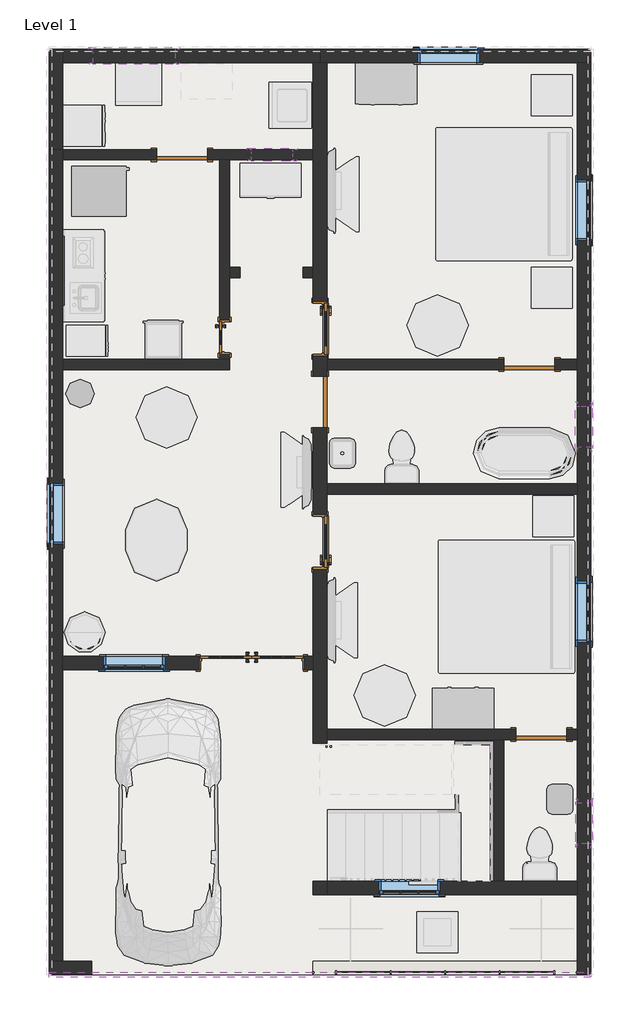
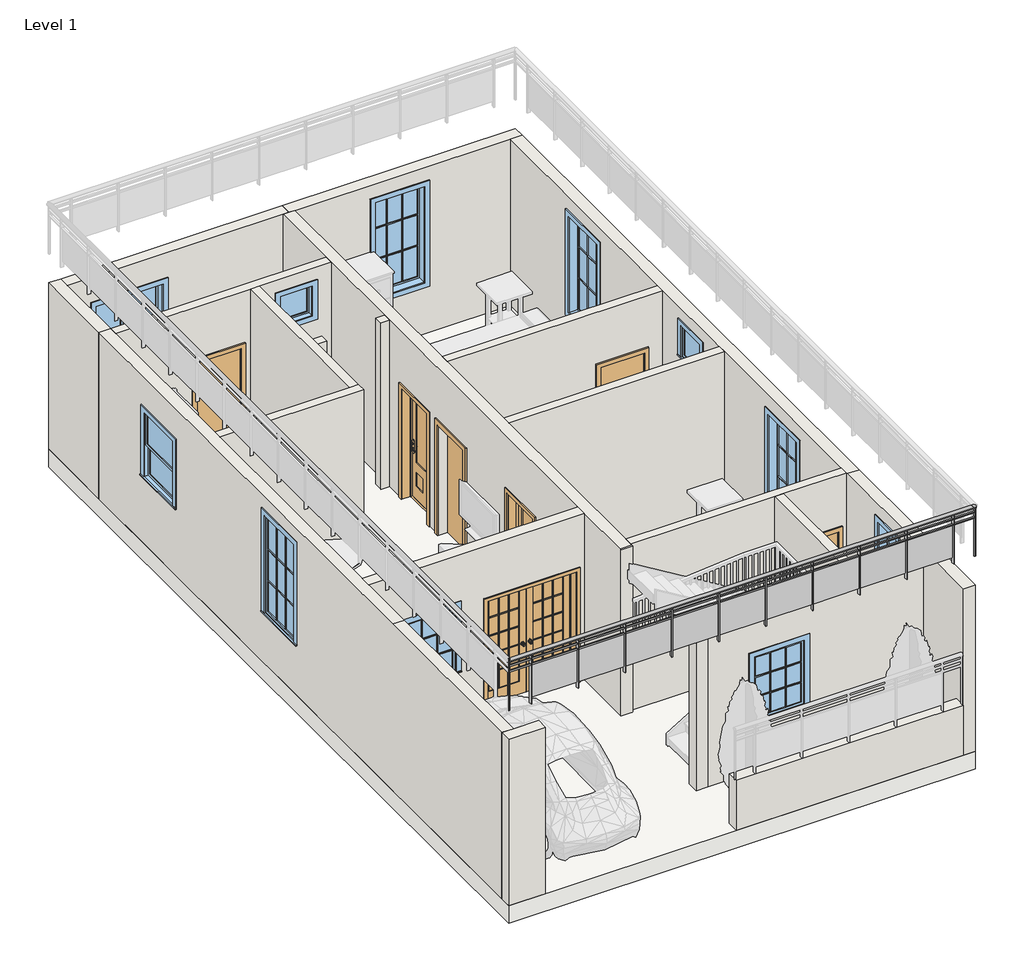
# One storey, part 1 of 3: 20 walls, 11 windows, 8 doors, 1 railing, 1 slab.
"""IFC4 building model written with IfcOpenShell, lengths in millimetres."""

from ifc_helpers import new_model, si_unit, point, frame, origin, origin_with_axes, place, context, project, spatial, polyline, ellipse_curve, trimmed, outline, extrude, faceted_brep, transform, mapped, element, save
from ifc_brep_helpers import plane_surface, extruded_surface, advanced_brep
from components import door_41326d50, door_ad59dcae, door_9d00318c, door_059bf842, door_059fdd7e, door_255cab33, door_53b1b562, window_29c06734, window_8b323df3, window_0862ab64, window_31198920, window_e41d21a6, window_3d781103

model = new_model("IFC4")

# Units and contexts
model_context = context("Model", 3, world=origin())
ifc_project = project(units=[si_unit("LENGTHUNIT", "METRE", prefix="MILLI")], contexts=[model_context])

# Site, building, storey
site = spatial("IfcSite", under=ifc_project)
building = spatial("IfcBuilding", under=site)
storey = spatial("IfcBuildingStorey", under=building, Name="Level 1", Elevation=0.0)

# Doors
placement = place(None, origin())
door_shape = door_41326d50(model_context)
element("IfcDoor", 1, ObjectType="30\" x 80\"", at=placement, inside=storey, context=model_context, shape_type="MappedRepresentation", body=[
    mapped(door_shape, transform((-8535.4123398, 7546.9033005, 0.0), x_axis=(0.0, 1.0, 0.0), y_axis=(-1.0, 0.0, 0.0), z_axis=(0.0, 0.0, 1.0))),
])
door_2_shape = door_ad59dcae(model_context)
element("IfcDoor", 2, ObjectType="30\" x 80\"", at=placement, inside=storey, context=model_context, shape_type="MappedRepresentation", body=[
    mapped(door_2_shape, transform((-8535.4123398, 4371.9033005, 0.0), x_axis=(0.0, -1.0, 0.0), y_axis=(1.0, 0.0, 0.0), z_axis=(0.0, 0.0, 1.0))),
])
door_3_shape = door_9d00318c(model_context)
element("IfcDoor", 3, ObjectType="Door-Interior-Double-Full Glass-Wood : 60\" x 80\"", at=placement, inside=storey, context=model_context, shape_type="MappedRepresentation", body=[
    mapped(door_3_shape, transform((-9554.5873398, 2571.6783005, 0.0), x_axis=(1.0, 0.0, 0.0), y_axis=(0.0, 1.0, 0.0), z_axis=(0.0, 0.0, 1.0))),
])
door_4_shape = door_059bf842(model_context)
element("IfcDoor", 4, ObjectType="Door-Interior-Single-Full Glass-Wood : 18\" x 80\"", at=placement, inside=storey, context=model_context, shape_type="MappedRepresentation", body=[
    mapped(door_4_shape, transform((-9964.1623398, 7419.9033005, 0.0), x_axis=(0.0, -1.0, 0.0), y_axis=(1.0, 0.0, 0.0), z_axis=(0.0, 0.0, 1.0))),
])
door_5_shape = door_059fdd7e(model_context)
element("IfcDoor", 5, ObjectType="Single-Flush : 30\" x 80\"", at=placement, inside=storey, context=model_context, shape_type="MappedRepresentation", body=[
    mapped(door_5_shape, transform((-5236.5873398, 1501.7033005, 0.0), x_axis=(-1.0, 0.0, 0.0), y_axis=(0.0, -1.0, 0.0), z_axis=(0.0, 0.0, 1.0))),
])
door_6_shape = door_255cab33(model_context)
element("IfcDoor", 6, ObjectType="Single-Flush : 30\" x 80\"", at=placement, inside=storey, context=model_context, shape_type="MappedRepresentation", body=[
    mapped(door_6_shape, transform((-5414.3873398, 7013.5033005, 0.0), x_axis=(1.0, 0.0, 0.0), y_axis=(0.0, 1.0, 0.0), z_axis=(0.0, 0.0, 1.0))),
])
element("IfcDoor", 7, ObjectType="Single-Flush : 30\" x 80\"", at=placement, inside=storey, context=model_context, shape_type="MappedRepresentation", body=[
    mapped(door_6_shape, transform((-10595.9873398, 10137.7033005, 0.0), x_axis=(1.0, 0.0, 0.0), y_axis=(0.0, 1.0, 0.0), z_axis=(0.0, 0.0, 1.0))),
])
door_7_shape = door_53b1b562(model_context)
element("IfcDoor", 8, ObjectType="Single-Flush : 30\" x 80\"", at=placement, inside=storey, context=model_context, shape_type="MappedRepresentation", body=[
    mapped(door_7_shape, transform((-8538.5873398, 6454.7033005, 0.0), x_axis=(0.0, 1.0, 0.0), y_axis=(-1.0, 0.0, 0.0), z_axis=(0.0, 0.0, 1.0))),
])

# Railing
element("IfcRailing", 9, ObjectType="Glass Panel - Bottom Fill", at=placement, inside=storey, context=model_context, shape_type="SolidModel", body=[
    advanced_brep(
    [(-12577.1873398, -2041.5966995, 4495.8), (-12577.1873398, -2117.7966995, 4495.8), (-4499.9873398, -2041.5966995, 4495.8), (-4499.9873398, -2117.7966995, 4495.8)],
    [
        (0, 1, ellipse_curve(frame((-12577.1873398, -2079.6966995, 4495.8), z_axis=(-1.0, 0.0, 0.0), x_axis=(0.0, -1.0, 0.0)), 38.1, 28.575)),
        (1, 0, ellipse_curve(frame((-12577.1873398, -2079.6966995, 4495.8), z_axis=(-1.0, 0.0, 0.0), x_axis=(0.0, -1.0, 0.0)), 38.1, 28.575)),
        (2, 3, ellipse_curve(frame((-4499.9873398, -2079.6966995, 4495.8), z_axis=(1.0, 0.0, 0.0), x_axis=(0.0, -1.0, 0.0)), 38.1, 28.575)),
        (3, 2, ellipse_curve(frame((-4499.9873398, -2079.6966995, 4495.8), z_axis=(1.0, 0.0, 0.0), x_axis=(0.0, -1.0, 0.0)), 38.1, 28.575)),
        (0, 2),
        (3, 1),
    ],
    [
        plane_surface(frame((-12577.1873398, -2079.6966995, 4495.8), z_axis=(-1.0, 0.0, 0.0), x_axis=(0.0, 1.0, 0.0))),
        plane_surface(frame((-4499.9873398, -2079.6966995, 4495.8), z_axis=(1.0, 0.0, 0.0), x_axis=(0.0, 1.0, 0.0))),
        extruded_surface(trimmed(ellipse_curve(frame((-4499.9873398, -2079.6966995, 4495.8), z_axis=(-1.0, 0.0, 0.0), x_axis=(0.0, -1.0, 0.0)), 38.1, 28.575), [point((-4499.9873398, -2041.5966995, 4495.8))], [point((-4499.9873398, -2117.7966995, 4495.8))], True, "CARTESIAN"), (-8077.200000000001, 0.0, 0.0), 8077.200000000001),
        extruded_surface(trimmed(ellipse_curve(frame((-4499.9873398, -2079.6966995, 4495.8), z_axis=(-1.0, 0.0, 0.0), x_axis=(0.0, -1.0, 0.0)), 38.1, 28.575), [point((-4499.9873398, -2117.7966995, 4495.8))], [point((-4499.9873398, -2041.5966995, 4495.8))], True, "CARTESIAN"), (-8077.200000000001, 0.0, 0.0), 8077.200000000001),
    ],
    [
        (0, [[1, 2]]),
        (1, [[3, 4]]),
        (2, [[-1, 5, -4, 6]]),
        (3, [[-2, -6, -3, -5]]),
    ],
),
    extrude(outline(polyline([(-12577.1873398, -2092.3966995), (-12577.1873398, -2066.9966995), (-4499.9873398, -2066.9966995), (-4499.9873398, -2092.3966995), (-12577.1873398, -2092.3966995)])), frame((0.0, 0.0, 4381.5), z_axis=(0.0, 0.0, 1.0), x_axis=(1.0, 0.0, 0.0)), (0.0, 0.0, 1.0), 25.4),
    extrude(outline(polyline([(-12577.1873398, -2092.3966995), (-12577.1873398, -2066.9966995), (-4499.9873398, -2066.9966995), (-4499.9873398, -2092.3966995), (-12577.1873398, -2092.3966995)])), frame((0.0, 0.0, 4279.9), z_axis=(0.0, 0.0, 1.0), x_axis=(1.0, 0.0, 0.0)), (0.0, 0.0, 1.0), 25.4),
    extrude(outline(polyline([(-4887.3373398, -2105.0966995), (-4887.3373398, -2054.2966995), (-4874.6373398, -2054.2966995), (-4874.6373398, -2105.0966995), (-4887.3373398, -2105.0966995)])), frame((0.0, 0.0, 3581.4), z_axis=(0.0, 0.0, 1.0), x_axis=(1.0, 0.0, 0.0)), (0.0, 0.0, 1.0), 885.6788223),
    extrude(outline(polyline([(-5693.7873398, -2073.1615425), (-4880.9873398, -2073.1615425), (-4880.9873398, -2079.5115425), (-5693.7873398, -2079.5115425), (-5693.7873398, -2073.1615425)])), frame((0.0, 0.0, 3683.0), z_axis=(0.0, 0.0, 1.0), x_axis=(1.0, 0.0, 0.0)), (0.0, 0.0, 1.0), 596.9),
    extrude(outline(polyline([(-5700.1373398, -2105.0966995), (-5700.1373398, -2054.2966995), (-5687.4373398, -2054.2966995), (-5687.4373398, -2105.0966995), (-5700.1373398, -2105.0966995)])), frame((0.0, 0.0, 3581.4), z_axis=(0.0, 0.0, 1.0), x_axis=(1.0, 0.0, 0.0)), (0.0, 0.0, 1.0), 885.6788223),
    extrude(outline(polyline([(-6506.5873398, -2073.1615425), (-5693.7873398, -2073.1615425), (-5693.7873398, -2079.5115425), (-6506.5873398, -2079.5115425), (-6506.5873398, -2073.1615425)])), frame((0.0, 0.0, 3683.0), z_axis=(0.0, 0.0, 1.0), x_axis=(1.0, 0.0, 0.0)), (0.0, 0.0, 1.0), 596.9),
    extrude(outline(polyline([(-6512.9373398, -2105.0966995), (-6512.9373398, -2054.2966995), (-6500.2373398, -2054.2966995), (-6500.2373398, -2105.0966995), (-6512.9373398, -2105.0966995)])), frame((0.0, 0.0, 3581.4), z_axis=(0.0, 0.0, 1.0), x_axis=(1.0, 0.0, 0.0)), (0.0, 0.0, 1.0), 885.6788223),
    extrude(outline(polyline([(-7319.3873398, -2073.1615425), (-6506.5873398, -2073.1615425), (-6506.5873398, -2079.5115425), (-7319.3873398, -2079.5115425), (-7319.3873398, -2073.1615425)])), frame((0.0, 0.0, 3683.0), z_axis=(0.0, 0.0, 1.0), x_axis=(1.0, 0.0, 0.0)), (0.0, 0.0, 1.0), 596.9),
    extrude(outline(polyline([(-7325.7373398, -2105.0966995), (-7325.7373398, -2054.2966995), (-7313.0373398, -2054.2966995), (-7313.0373398, -2105.0966995), (-7325.7373398, -2105.0966995)])), frame((0.0, 0.0, 3581.4), z_axis=(0.0, 0.0, 1.0), x_axis=(1.0, 0.0, 0.0)), (0.0, 0.0, 1.0), 885.6788223),
    extrude(outline(polyline([(-8132.1873398, -2073.1615425), (-7319.3873398, -2073.1615425), (-7319.3873398, -2079.5115425), (-8132.1873398, -2079.5115425), (-8132.1873398, -2073.1615425)])), frame((0.0, 0.0, 3683.0), z_axis=(0.0, 0.0, 1.0), x_axis=(1.0, 0.0, 0.0)), (0.0, 0.0, 1.0), 596.9),
    extrude(outline(polyline([(-8138.5373398, -2105.0966995), (-8138.5373398, -2054.2966995), (-8125.8373398, -2054.2966995), (-8125.8373398, -2105.0966995), (-8138.5373398, -2105.0966995)])), frame((0.0, 0.0, 3581.4), z_axis=(0.0, 0.0, 1.0), x_axis=(1.0, 0.0, 0.0)), (0.0, 0.0, 1.0), 885.6788223),
    extrude(outline(polyline([(-8944.9873398, -2073.1615425), (-8132.1873398, -2073.1615425), (-8132.1873398, -2079.5115425), (-8944.9873398, -2079.5115425), (-8944.9873398, -2073.1615425)])), frame((0.0, 0.0, 3683.0), z_axis=(0.0, 0.0, 1.0), x_axis=(1.0, 0.0, 0.0)), (0.0, 0.0, 1.0), 596.9),
    extrude(outline(polyline([(-8951.3373398, -2105.0966995), (-8951.3373398, -2054.2966995), (-8938.6373398, -2054.2966995), (-8938.6373398, -2105.0966995), (-8951.3373398, -2105.0966995)])), frame((0.0, 0.0, 3581.4), z_axis=(0.0, 0.0, 1.0), x_axis=(1.0, 0.0, 0.0)), (0.0, 0.0, 1.0), 885.6788223),
    extrude(outline(polyline([(-9757.7873398, -2073.1615425), (-8944.9873398, -2073.1615425), (-8944.9873398, -2079.5115425), (-9757.7873398, -2079.5115425), (-9757.7873398, -2073.1615425)])), frame((0.0, 0.0, 3683.0), z_axis=(0.0, 0.0, 1.0), x_axis=(1.0, 0.0, 0.0)), (0.0, 0.0, 1.0), 596.9),
    extrude(outline(polyline([(-9764.1373398, -2105.0966995), (-9764.1373398, -2054.2966995), (-9751.4373398, -2054.2966995), (-9751.4373398, -2105.0966995), (-9764.1373398, -2105.0966995)])), frame((0.0, 0.0, 3581.4), z_axis=(0.0, 0.0, 1.0), x_axis=(1.0, 0.0, 0.0)), (0.0, 0.0, 1.0), 885.6788223),
    extrude(outline(polyline([(-10570.5873398, -2073.1615425), (-9757.7873398, -2073.1615425), (-9757.7873398, -2079.5115425), (-10570.5873398, -2079.5115425), (-10570.5873398, -2073.1615425)])), frame((0.0, 0.0, 3683.0), z_axis=(0.0, 0.0, 1.0), x_axis=(1.0, 0.0, 0.0)), (0.0, 0.0, 1.0), 596.9),
    extrude(outline(polyline([(-10576.9373398, -2105.0966995), (-10576.9373398, -2054.2966995), (-10564.2373398, -2054.2966995), (-10564.2373398, -2105.0966995), (-10576.9373398, -2105.0966995)])), frame((0.0, 0.0, 3581.4), z_axis=(0.0, 0.0, 1.0), x_axis=(1.0, 0.0, 0.0)), (0.0, 0.0, 1.0), 885.6788223),
    extrude(outline(polyline([(-11383.3873398, -2073.1615425), (-10570.5873398, -2073.1615425), (-10570.5873398, -2079.5115425), (-11383.3873398, -2079.5115425), (-11383.3873398, -2073.1615425)])), frame((0.0, 0.0, 3683.0), z_axis=(0.0, 0.0, 1.0), x_axis=(1.0, 0.0, 0.0)), (0.0, 0.0, 1.0), 596.9),
    extrude(outline(polyline([(-11389.7373398, -2105.0966995), (-11389.7373398, -2054.2966995), (-11377.0373398, -2054.2966995), (-11377.0373398, -2105.0966995), (-11389.7373398, -2105.0966995)])), frame((0.0, 0.0, 3581.4), z_axis=(0.0, 0.0, 1.0), x_axis=(1.0, 0.0, 0.0)), (0.0, 0.0, 1.0), 885.6788223),
    extrude(outline(polyline([(-12196.1873398, -2073.1615425), (-11383.3873398, -2073.1615425), (-11383.3873398, -2079.5115425), (-12196.1873398, -2079.5115425), (-12196.1873398, -2073.1615425)])), frame((0.0, 0.0, 3683.0), z_axis=(0.0, 0.0, 1.0), x_axis=(1.0, 0.0, 0.0)), (0.0, 0.0, 1.0), 596.9),
    extrude(outline(polyline([(-12202.5373398, -2105.0966995), (-12202.5373398, -2054.2966995), (-12189.8373398, -2054.2966995), (-12189.8373398, -2105.0966995), (-12202.5373398, -2105.0966995)])), frame((0.0, 0.0, 3581.4), z_axis=(0.0, 0.0, 1.0), x_axis=(1.0, 0.0, 0.0)), (0.0, 0.0, 1.0), 885.6788223),
    extrude(outline(polyline([(-4512.6873398, -2089.2216995), (-4512.6873398, -2070.1716995), (-4493.6373398, -2070.1716995), (-4493.6373398, -2089.2216995), (-4512.6873398, -2089.2216995)])), frame((0.0, 0.0, 3581.4), z_axis=(0.0, 0.0, 1.0), x_axis=(1.0, 0.0, 0.0)), (0.0, 0.0, 1.0), 885.6788223),
    extrude(outline(polyline([(-12583.5373398, -2089.2216995), (-12583.5373398, -2070.1716995), (-12564.4873398, -2070.1716995), (-12564.4873398, -2089.2216995), (-12583.5373398, -2089.2216995)])), frame((0.0, 0.0, 3581.4), z_axis=(0.0, 0.0, 1.0), x_axis=(1.0, 0.0, 0.0)), (0.0, 0.0, 1.0), 885.6788223),
])

# Slab
element("IfcSlab", 10, at=placement, inside=storey, context=model_context, shape_type="SweptSolid", body=[
    extrude(outline(polyline([(-4499.9873398, 11712.5033005), (-4499.9873398, -2079.6966995), (-12577.1873398, -2079.6966995), (-12577.1873398, 11712.5033005), (-4499.9873398, 11712.5033005)])), frame((0.0, 0.0, -323.85), z_axis=(0.0, 0.0, 1.0), x_axis=(1.0, 0.0, 0.0)), (0.0, 0.0, 1.0), 323.85),
])

# Walls
element("IfcWall", 11, ObjectType="Generic - 8\"", at=placement, inside=storey, context=model_context, shape_type="Brep", body=[
    faceted_brep([(-4703.1873398, 11509.3033005, 0.0), (-4703.1873398, 7089.7033005, 0.0), (-4703.1873398, 6937.3033005, 0.0), (-4703.1873398, 5235.5033005, 0.0), (-4703.1873398, 5083.1033005, 0.0), (-4703.1873398, 1577.9033005, 0.0), (-4703.1873398, 1425.5033005, 0.0), (-4703.1873398, -682.6966995, 0.0), (-4703.1873398, -885.8966995, 0.0), (-4703.1873398, -1876.4966995, 0.0), (-4703.1873398, -2079.6966995, 0.0), (-4703.1873398, -2079.6966995, 914.4), (-4703.1873398, -2079.6966995, 3048.0), (-4703.1873398, -885.8966995, 3048.0), (-4703.1873398, -682.6966995, 3048.0), (-4703.1873398, 1400.1033005, 3048.0), (-4703.1873398, 1425.5033005, 3048.0), (-4703.1873398, 1577.9033005, 3048.0), (-4703.1873398, 5083.1033005, 3048.0), (-4703.1873398, 5235.5033005, 3048.0), (-4703.1873398, 6937.3033005, 3048.0), (-4703.1873398, 7089.7033005, 3048.0), (-4703.1873398, 11509.3033005, 3048.0), (-4703.1873398, 2873.3033005, 2743.2), (-4703.1873398, 2873.3033005, 914.4), (-4703.1873398, 3787.7033005, 914.4), (-4703.1873398, 3787.7033005, 2743.2), (-4703.1873398, 8855.0033005, 2743.2), (-4703.1873398, 8855.0033005, 914.4), (-4703.1873398, 9769.4033005, 914.4), (-4703.1873398, 9769.4033005, 2743.2), (-4703.1873398, -123.8966995, 2768.6), (-4703.1873398, -123.8966995, 2159.0), (-4703.1873398, 485.7033005, 2159.0), (-4703.1873398, 485.7033005, 2768.6), (-4703.1873398, 6391.2033005, 2768.6), (-4703.1873398, 5781.6033005, 2768.6), (-4703.1873398, 5781.6033005, 2159.0), (-4703.1873398, 6391.2033005, 2159.0), (-4499.9873398, 11509.3033005, 0.0), (-4499.9873398, 11509.3033005, 3048.0), (-4499.9873398, 1400.1033005, 3048.0), (-4499.9873398, -2079.6966995, 3048.0), (-4499.9873398, -2079.6966995, 0.0), (-4499.9873398, 2873.3033005, 2743.2), (-4499.9873398, 3787.7033005, 2743.2), (-4499.9873398, 3787.7033005, 914.4), (-4499.9873398, 2873.3033005, 914.4), (-4499.9873398, 8855.0033005, 2743.2), (-4499.9873398, 9769.4033005, 2743.2), (-4499.9873398, 9769.4033005, 914.4), (-4499.9873398, 8855.0033005, 914.4), (-4499.9873398, -123.8966995, 2768.6), (-4499.9873398, 485.7033005, 2768.6), (-4499.9873398, 485.7033005, 2159.0), (-4499.9873398, -123.8966995, 2159.0), (-4499.9873398, 6391.2033005, 2768.6), (-4499.9873398, 6391.2033005, 2159.0), (-4499.9873398, 5781.6033005, 2159.0), (-4499.9873398, 5781.6033005, 2768.6)], [[[0, 1, 2, 3, 4, 5, 6, 7, 8, 9, 10, 11, 12, 13, 14, 15, 16, 17, 18, 19, 20, 21, 22], [23, 24, 25, 26], [27, 28, 29, 30], [31, 32, 33, 34], [35, 36, 37, 38]], [[39, 40, 41, 42, 43], [44, 45, 46, 47], [48, 49, 50, 51], [52, 53, 54, 55], [56, 57, 58, 59]], [[10, 9, 8, 7, 6, 5, 4, 3, 2, 1, 0, 39, 43]], [[0, 22, 40, 39]], [[12, 11, 10, 43, 42]], [[15, 14, 13, 12, 42, 41]], [[22, 21, 20, 19, 18, 17, 16, 15, 41, 40]], [[24, 23, 44, 47]], [[25, 24, 47, 46]], [[26, 25, 46, 45]], [[23, 26, 45, 44]], [[28, 27, 48, 51]], [[29, 28, 51, 50]], [[30, 29, 50, 49]], [[27, 30, 49, 48]], [[32, 31, 52, 55]], [[33, 32, 55, 54]], [[34, 33, 54, 53]], [[31, 34, 53, 52]], [[57, 56, 35, 38]], [[58, 57, 38, 37]], [[59, 58, 37, 36]], [[56, 59, 36, 35]]]),
])
element("IfcWall", 12, ObjectType="Generic - 8\"", at=placement, inside=storey, context=model_context, shape_type="SweptSolid", body=[
    extrude(outline(polyline([(-8640.1873398, -1876.4966995), (-4703.1873398, -1876.4966995), (-4703.1873398, -2079.6966995), (-8640.1873398, -2079.6966995), (-8640.1873398, -1876.4966995)])), origin_with_axes(), (0.0, 0.0, 1.0), 914.4),
])
element("IfcWall", 13, ObjectType="Generic - 8\"", at=placement, inside=storey, context=model_context, shape_type="Brep", body=[
    faceted_brep([(-12373.9873398, -1876.4966995, 0.0), (-12373.9873398, 2466.9033005, 0.0), (-12373.9873398, 2670.1033005, 0.0), (-12373.9873398, 6937.3033005, 0.0), (-12373.9873398, 7089.7033005, 0.0), (-12373.9873398, 10061.5033005, 0.0), (-12373.9873398, 10213.9033005, 0.0), (-12373.9873398, 10213.9033005, 3048.0), (-12373.9873398, 10061.5033005, 3048.0), (-12373.9873398, 7089.7033005, 3048.0), (-12373.9873398, 6937.3033005, 3048.0), (-12373.9873398, 2670.1033005, 3048.0), (-12373.9873398, 2466.9033005, 3048.0), (-12373.9873398, 1400.1033005, 3048.0), (-12373.9873398, -1876.4966995, 3048.0), (-12373.9873398, 5248.2033005, 2743.2), (-12373.9873398, 5248.2033005, 914.4), (-12373.9873398, 4333.8033005, 914.4), (-12373.9873398, 4333.8033005, 2743.2), (-12373.9873398, 8867.7033005, 2438.4), (-12373.9873398, 8867.7033005, 1219.2), (-12373.9873398, 7953.3033005, 1219.2), (-12373.9873398, 7953.3033005, 2438.4), (-12577.1873398, -1876.4966995, 0.0), (-12577.1873398, -1876.4966995, 3048.0), (-12577.1873398, 1400.1033005, 3048.0), (-12577.1873398, 10213.9033005, 3048.0), (-12577.1873398, 10213.9033005, 0.0), (-12577.1873398, 5248.2033005, 2743.2), (-12577.1873398, 4333.8033005, 2743.2), (-12577.1873398, 4333.8033005, 914.4), (-12577.1873398, 5248.2033005, 914.4), (-12577.1873398, 8867.7033005, 2438.4), (-12577.1873398, 7953.3033005, 2438.4), (-12577.1873398, 7953.3033005, 1219.2), (-12577.1873398, 8867.7033005, 1219.2)], [[[0, 1, 2, 3, 4, 5, 6, 7, 8, 9, 10, 11, 12, 13, 14], [15, 16, 17, 18], [19, 20, 21, 22]], [[23, 24, 25, 26, 27], [28, 29, 30, 31], [32, 33, 34, 35]], [[6, 5, 4, 3, 2, 1, 0, 23, 27]], [[7, 6, 27, 26]], [[0, 14, 24, 23]], [[14, 13, 25, 24]], [[13, 12, 11, 10, 9, 8, 7, 26, 25]], [[16, 15, 28, 31]], [[17, 16, 31, 30]], [[18, 17, 30, 29]], [[15, 18, 29, 28]], [[20, 19, 32, 35]], [[21, 20, 35, 34]], [[22, 21, 34, 33]], [[19, 22, 33, 32]]]),
])
element("IfcWall", 14, ObjectType="Generic - 8\"", at=placement, inside=storey, context=model_context, shape_type="Brep", body=[
    faceted_brep([(-8640.1873398, 1374.7033005, 0.0), (-8640.1873398, 1374.7033005, 3048.0), (-8640.1873398, 1400.1033005, 3048.0), (-8640.1873398, 2466.9033005, 3048.0), (-8640.1873398, 2670.1033005, 3048.0), (-8640.1873398, 8308.9033005, 3048.0), (-8640.1873398, 8461.3033005, 3048.0), (-8640.1873398, 10061.5033005, 3048.0), (-8640.1873398, 10213.9033005, 3048.0), (-8640.1873398, 11509.3033005, 3048.0), (-8640.1873398, 11509.3033005, 0.0), (-8640.1873398, 10213.9033005, 0.0), (-8640.1873398, 10061.5033005, 0.0), (-8640.1873398, 8461.3033005, 0.0), (-8640.1873398, 8308.9033005, 0.0), (-8640.1873398, 7953.3033005, 0.0), (-8640.1873398, 7953.3033005, 2057.4), (-8640.1873398, 7140.5033005, 2057.4), (-8640.1873398, 7140.5033005, 0.0), (-8640.1873398, 6835.7033005, 0.0), (-8640.1873398, 6835.7033005, 2032.0), (-8640.1873398, 6073.7033005, 2032.0), (-8640.1873398, 6073.7033005, 0.0), (-8640.1873398, 4778.3033005, 0.0), (-8640.1873398, 4778.3033005, 2057.4), (-8640.1873398, 3965.5033005, 2057.4), (-8640.1873398, 3965.5033005, 0.0), (-8640.1873398, 2670.1033005, 0.0), (-8640.1873398, 2466.9033005, 0.0), (-8436.9873398, 1374.7033005, 3048.0), (-8436.9873398, 1374.7033005, 0.0), (-8436.9873398, 1425.5033005, 0.0), (-8436.9873398, 1577.9033005, 0.0), (-8436.9873398, 3965.5033005, 0.0), (-8436.9873398, 3965.5033005, 2057.4), (-8436.9873398, 4778.3033005, 2057.4), (-8436.9873398, 4778.3033005, 0.0), (-8436.9873398, 5083.1033005, 0.0), (-8436.9873398, 5235.5033005, 0.0), (-8436.9873398, 6073.7033005, 0.0), (-8436.9873398, 6073.7033005, 2032.0), (-8436.9873398, 6835.7033005, 2032.0), (-8436.9873398, 6835.7033005, 0.0), (-8436.9873398, 6937.3033005, 0.0), (-8436.9873398, 7089.7033005, 0.0), (-8436.9873398, 7140.5033005, 0.0), (-8436.9873398, 7140.5033005, 2057.4), (-8436.9873398, 7953.3033005, 2057.4), (-8436.9873398, 7953.3033005, 0.0), (-8436.9873398, 11509.3033005, 0.0), (-8436.9873398, 11509.3033005, 3048.0), (-8436.9873398, 7089.7033005, 3048.0), (-8436.9873398, 6937.3033005, 3048.0), (-8436.9873398, 5235.5033005, 3048.0), (-8436.9873398, 5083.1033005, 3048.0), (-8436.9873398, 1577.9033005, 3048.0), (-8436.9873398, 1425.5033005, 3048.0), (-8436.9873398, 1400.1033005, 3048.0), (-8538.5873398, 11509.3033005, 0.0), (-8538.5873398, 11509.3033005, 3048.0)], [[[0, 1, 2, 3, 4, 5, 6, 7, 8, 9, 10, 11, 12, 13, 14, 15, 16, 17, 18, 19, 20, 21, 22, 23, 24, 25, 26, 27, 28]], [[29, 30, 31, 32, 33, 34, 35, 36, 37, 38, 39, 40, 41, 42, 43, 44, 45, 46, 47, 48, 49, 50, 51, 52, 53, 54, 55, 56, 57]], [[30, 0, 28, 27, 26, 33, 32, 31]], [[48, 15, 14, 13, 12, 11, 10, 58, 49]], [[18, 45, 44, 43, 42, 19]], [[22, 39, 38, 37, 36, 23]], [[1, 0, 30, 29]], [[1, 29, 57, 2]], [[9, 8, 7, 6, 5, 4, 3, 2, 57, 56, 55, 54, 53, 52, 51, 50, 59]], [[47, 16, 15, 48]], [[16, 47, 46, 17]], [[17, 46, 45, 18]], [[20, 19, 42, 41]], [[21, 20, 41, 40]], [[22, 21, 40, 39]], [[10, 9, 59, 50, 49, 58]], [[25, 34, 33, 26]], [[34, 25, 24, 35]], [[35, 24, 23, 36]]]),
])
element("IfcWall", 15, ObjectType="Generic - 8\"", at=placement, inside=storey, context=model_context, shape_type="Brep", body=[
    faceted_brep([(-4703.1873398, -682.6966995, 0.0), (-5795.3873398, -682.6966995, 0.0), (-5947.7873398, -682.6966995, 0.0), (-8436.9873398, -682.6966995, 0.0), (-8436.9873398, -682.6966995, 3048.0), (-5947.7873398, -682.6966995, 3048.0), (-5795.3873398, -682.6966995, 3048.0), (-4703.1873398, -682.6966995, 3048.0), (-7662.2873398, -682.6966995, 2133.6), (-7662.2873398, -682.6966995, 914.4), (-6747.8873398, -682.6966995, 914.4), (-6747.8873398, -682.6966995, 2133.6), (-4703.1873398, -885.8966995, 0.0), (-4703.1873398, -885.8966995, 3048.0), (-8436.9873398, -885.8966995, 3048.0), (-8436.9873398, -885.8966995, 0.0), (-7662.2873398, -885.8966995, 2133.6), (-6747.8873398, -885.8966995, 2133.6), (-6747.8873398, -885.8966995, 914.4), (-7662.2873398, -885.8966995, 914.4)], [[[0, 1, 2, 3, 4, 5, 6, 7], [8, 9, 10, 11]], [[12, 13, 14, 15], [16, 17, 18, 19]], [[3, 2, 1, 0, 12, 15]], [[0, 7, 13, 12]], [[4, 3, 15, 14]], [[7, 6, 5, 4, 14, 13]], [[9, 8, 16, 19]], [[10, 9, 19, 18]], [[11, 10, 18, 17]], [[8, 11, 17, 16]]]),
])
element("IfcWall", 16, ObjectType="Generic - 8\"", at=placement, inside=storey, context=model_context, shape_type="SweptSolid", body=[
    extrude(outline(polyline([(3048.0, -12373.9873398), (0.0, -12373.9873398), (0.0, -10341.9873398), (2057.4, -10341.9873398), (2057.4, -8767.1873398), (0.0, -8767.1873398), (0.0, -8640.1873398), (3048.0, -8640.1873398), (3048.0, -12373.9873398)]), holes=[polyline([(2133.6, -11764.3873398), (2133.6, -10849.9873398), (914.4, -10849.9873398), (914.4, -11764.3873398), (2133.6, -11764.3873398)])]), frame((0.0, 2466.9033005, 0.0), z_axis=(0.0, 1.0, 0.0), x_axis=(0.0, 0.0, 1.0)), (0.0, 0.0, 1.0), 203.2),
])
element("IfcWall", 17, ObjectType="Generic - 8\"", at=placement, inside=storey, context=model_context, shape_type="SweptSolid", body=[
    extrude(outline(polyline([(-8640.1873398, -885.8966995), (-8640.1873398, -682.6966995), (-8436.9873398, -682.6966995), (-8436.9873398, -885.8966995), (-8640.1873398, -885.8966995)])), origin_with_axes(), (0.0, 0.0, 1.0), 3048.0),
])
element("IfcWall", 18, ObjectType="Generic - 8\"", at=placement, inside=storey, context=model_context, shape_type="Brep", body=[
    faceted_brep([(-12373.9873398, 11509.3033005, 0.0), (-8640.1873398, 11509.3033005, 0.0), (-8538.5873398, 11509.3033005, 0.0), (-8538.5873398, 11509.3033005, 3048.0), (-8640.1873398, 11509.3033005, 3048.0), (-12373.9873398, 11509.3033005, 3048.0), (-10697.5873398, 11509.3033005, 2540.0), (-10697.5873398, 11509.3033005, 1320.8), (-11916.7873398, 11509.3033005, 1320.8), (-11916.7873398, 11509.3033005, 2540.0), (-12373.9873398, 11712.5033005, 0.0), (-12373.9873398, 11712.5033005, 3048.0), (-8538.5873398, 11712.5033005, 3048.0), (-8538.5873398, 11712.5033005, 0.0), (-10697.5873398, 11712.5033005, 2540.0), (-11916.7873398, 11712.5033005, 2540.0), (-11916.7873398, 11712.5033005, 1320.8), (-10697.5873398, 11712.5033005, 1320.8)], [[[0, 1, 2, 3, 4, 5], [6, 7, 8, 9]], [[10, 11, 12, 13], [14, 15, 16, 17]], [[2, 1, 0, 10, 13]], [[3, 2, 13, 12]], [[5, 4, 3, 12, 11]], [[0, 5, 11, 10]], [[7, 6, 14, 17]], [[8, 7, 17, 16]], [[9, 8, 16, 15]], [[6, 9, 15, 14]]]),
])
element("IfcWall", 19, ObjectType="Generic - 8\"", at=placement, inside=storey, context=model_context, shape_type="Brep", body=[
    faceted_brep([(-8538.5873398, 11509.3033005, 0.0), (-8436.9873398, 11509.3033005, 0.0), (-4703.1873398, 11509.3033005, 0.0), (-4499.9873398, 11509.3033005, 0.0), (-4499.9873398, 11509.3033005, 3048.0), (-4703.1873398, 11509.3033005, 3048.0), (-8436.9873398, 11509.3033005, 3048.0), (-8538.5873398, 11509.3033005, 3048.0), (-6163.6873398, 11509.3033005, 2743.2), (-6163.6873398, 11509.3033005, 914.4), (-7078.0873398, 11509.3033005, 914.4), (-7078.0873398, 11509.3033005, 2743.2), (-8538.5873398, 11712.5033005, 0.0), (-8538.5873398, 11712.5033005, 3048.0), (-4499.9873398, 11712.5033005, 3048.0), (-4499.9873398, 11712.5033005, 0.0), (-6163.6873398, 11712.5033005, 2743.2), (-7078.0873398, 11712.5033005, 2743.2), (-7078.0873398, 11712.5033005, 914.4), (-6163.6873398, 11712.5033005, 914.4)], [[[0, 1, 2, 3, 4, 5, 6, 7], [8, 9, 10, 11]], [[12, 13, 14, 15], [16, 17, 18, 19]], [[3, 2, 1, 0, 12, 15]], [[0, 7, 13, 12]], [[4, 3, 15, 14]], [[7, 6, 5, 4, 14, 13]], [[8, 11, 17, 16]], [[11, 10, 18, 17]], [[10, 9, 19, 18]], [[9, 8, 16, 19]]]),
])
element("IfcWall", 20, ObjectType="Generic - 8\"", at=placement, inside=storey, context=model_context, shape_type="Brep", body=[
    faceted_brep([(-12373.9873398, 10213.9033005, 0.0), (-12373.9873398, 11509.3033005, 0.0), (-12373.9873398, 11712.5033005, 0.0), (-12373.9873398, 11712.5033005, 3048.0), (-12373.9873398, 11509.3033005, 3048.0), (-12373.9873398, 10213.9033005, 3048.0), (-12577.1873398, 10213.9033005, 0.0), (-12577.1873398, 10213.9033005, 3048.0), (-12577.1873398, 11712.5033005, 3048.0), (-12577.1873398, 11712.5033005, 0.0)], [[[0, 1, 2, 3, 4, 5]], [[6, 7, 8, 9]], [[2, 1, 0, 6, 9]], [[0, 5, 7, 6]], [[3, 2, 9, 8]], [[5, 4, 3, 8, 7]]]),
])
element("IfcWall", 21, ObjectType="Generic - 8\"", at=placement, inside=storey, context=model_context, shape_type="Brep", body=[
    faceted_brep([(-11942.1873398, -1876.4966995, 0.0), (-12373.9873398, -1876.4966995, 0.0), (-12577.1873398, -1876.4966995, 0.0), (-12577.1873398, -1876.4966995, 3048.0), (-12373.9873398, -1876.4966995, 3048.0), (-11942.1873398, -1876.4966995, 3048.0), (-11942.1873398, -2079.6966995, 0.0), (-11942.1873398, -2079.6966995, 3048.0), (-12577.1873398, -2079.6966995, 3048.0), (-12577.1873398, -2079.6966995, 0.0)], [[[0, 1, 2, 3, 4, 5]], [[6, 7, 8, 9]], [[2, 1, 0, 6, 9]], [[0, 5, 7, 6]], [[3, 2, 9, 8]], [[5, 4, 3, 8, 7]]]),
])
element("IfcWall", 22, ObjectType="inner", at=placement, inside=storey, context=model_context, shape_type="Brep", body=[
    faceted_brep([(-10214.9873398, 10061.5033005, 2032.0), (-10214.9873398, 10061.5033005, 0.0), (-10037.1873398, 10061.5033005, 0.0), (-9884.7873398, 10061.5033005, 0.0), (-8640.1873398, 10061.5033005, 0.0), (-8640.1873398, 10061.5033005, 3048.0), (-9884.7873398, 10061.5033005, 3048.0), (-10037.1873398, 10061.5033005, 3048.0), (-12373.9873398, 10061.5033005, 3048.0), (-12373.9873398, 10061.5033005, 0.0), (-10976.9873398, 10061.5033005, 0.0), (-10976.9873398, 10061.5033005, 2032.0), (-8944.9873398, 10061.5033005, 2768.6), (-8944.9873398, 10061.5033005, 2159.0), (-9554.5873398, 10061.5033005, 2159.0), (-9554.5873398, 10061.5033005, 2768.6), (-8640.1873398, 10213.9033005, 0.0), (-10214.9873398, 10213.9033005, 0.0), (-10214.9873398, 10213.9033005, 2032.0), (-10976.9873398, 10213.9033005, 2032.0), (-10976.9873398, 10213.9033005, 0.0), (-12373.9873398, 10213.9033005, 0.0), (-12373.9873398, 10213.9033005, 3048.0), (-8640.1873398, 10213.9033005, 3048.0), (-8944.9873398, 10213.9033005, 2768.6), (-9554.5873398, 10213.9033005, 2768.6), (-9554.5873398, 10213.9033005, 2159.0), (-8944.9873398, 10213.9033005, 2159.0)], [[[0, 1, 2, 3, 4, 5, 6, 7, 8, 9, 10, 11], [12, 13, 14, 15]], [[16, 17, 18, 19, 20, 21, 22, 23], [24, 25, 26, 27]], [[10, 9, 21, 20]], [[4, 3, 2, 1, 17, 16]], [[9, 8, 22, 21]], [[5, 4, 16, 23]], [[8, 7, 6, 5, 23, 22]], [[18, 17, 1, 0]], [[19, 18, 0, 11]], [[20, 19, 11, 10]], [[13, 12, 24, 27]], [[14, 13, 27, 26]], [[15, 14, 26, 25]], [[12, 15, 25, 24]]]),
])
element("IfcWall", 23, ObjectType="inner", at=placement, inside=storey, context=model_context, shape_type="Brep", body=[
    faceted_brep([(-12373.9873398, 6937.3033005, 0.0), (-9884.7873398, 6937.3033005, 0.0), (-9884.7873398, 6937.3033005, 3048.0), (-12373.9873398, 6937.3033005, 3048.0), (-12373.9873398, 7089.7033005, 0.0), (-12373.9873398, 7089.7033005, 3048.0), (-10037.1873398, 7089.7033005, 3048.0), (-9884.7873398, 7089.7033005, 3048.0), (-9884.7873398, 7089.7033005, 0.0), (-10037.1873398, 7089.7033005, 0.0)], [[[0, 1, 2, 3]], [[4, 5, 6, 7, 8, 9]], [[1, 0, 4, 9, 8]], [[0, 3, 5, 4]], [[3, 2, 7, 6, 5]], [[2, 1, 8, 7]]]),
])
element("IfcWall", 24, ObjectType="inner", at=placement, inside=storey, context=model_context, shape_type="Brep", body=[
    faceted_brep([(-10037.1873398, 10061.5033005, 3048.0), (-10037.1873398, 10061.5033005, 0.0), (-10037.1873398, 7673.9033005, 0.0), (-10037.1873398, 7673.9033005, 2057.4), (-10037.1873398, 7165.9033005, 2057.4), (-10037.1873398, 7165.9033005, 0.0), (-10037.1873398, 7089.7033005, 0.0), (-10037.1873398, 7089.7033005, 3048.0), (-9884.7873398, 10061.5033005, 0.0), (-9884.7873398, 10061.5033005, 3048.0), (-9884.7873398, 8461.3033005, 3048.0), (-9884.7873398, 8308.9033005, 3048.0), (-9884.7873398, 7089.7033005, 3048.0), (-9884.7873398, 7089.7033005, 0.0), (-9884.7873398, 7165.9033005, 0.0), (-9884.7873398, 7165.9033005, 2057.4), (-9884.7873398, 7673.9033005, 2057.4), (-9884.7873398, 7673.9033005, 0.0), (-9884.7873398, 8308.9033005, 0.0), (-9884.7873398, 8461.3033005, 0.0)], [[[0, 1, 2, 3, 4, 5, 6, 7]], [[8, 9, 10, 11, 12, 13, 14, 15, 16, 17, 18, 19]], [[1, 8, 19, 18, 17, 2]], [[13, 6, 5, 14]], [[1, 0, 9, 8]], [[0, 7, 12, 11, 10, 9]], [[7, 6, 13, 12]], [[4, 15, 14, 5]], [[15, 4, 3, 16]], [[16, 3, 2, 17]]]),
])
element("IfcWall", 25, ObjectType="inner", at=placement, inside=storey, context=model_context, shape_type="SweptSolid", body=[
    extrude(outline(polyline([(-8792.5873398, 8461.3033005), (-8640.1873398, 8461.3033005), (-8640.1873398, 8308.9033005), (-8792.5873398, 8308.9033005), (-8792.5873398, 8461.3033005)])), origin_with_axes(), (0.0, 0.0, 1.0), 3048.0),
])
element("IfcWall", 26, ObjectType="inner", at=placement, inside=storey, context=model_context, shape_type="SweptSolid", body=[
    extrude(outline(polyline([(-8436.9873398, 5235.5033005), (-4703.1873398, 5235.5033005), (-4703.1873398, 5083.1033005), (-8436.9873398, 5083.1033005), (-8436.9873398, 5235.5033005)])), origin_with_axes(), (0.0, 0.0, 1.0), 3048.0),
])
element("IfcWall", 27, ObjectType="inner", at=placement, inside=storey, context=model_context, shape_type="Brep", body=[
    faceted_brep([(-5617.5873398, 1577.9033005, 2032.0), (-5617.5873398, 1577.9033005, 0.0), (-8436.9873398, 1577.9033005, 0.0), (-8436.9873398, 1577.9033005, 3048.0), (-4703.1873398, 1577.9033005, 3048.0), (-4703.1873398, 1577.9033005, 0.0), (-4855.5873398, 1577.9033005, 0.0), (-4855.5873398, 1577.9033005, 2032.0), (-8436.9873398, 1425.5033005, 0.0), (-5947.7873398, 1425.5033005, 0.0), (-5795.3873398, 1425.5033005, 0.0), (-5617.5873398, 1425.5033005, 0.0), (-5617.5873398, 1425.5033005, 2032.0), (-4855.5873398, 1425.5033005, 2032.0), (-4855.5873398, 1425.5033005, 0.0), (-4703.1873398, 1425.5033005, 0.0), (-4703.1873398, 1425.5033005, 3048.0), (-5795.3873398, 1425.5033005, 3048.0), (-5947.7873398, 1425.5033005, 3048.0), (-8436.9873398, 1425.5033005, 3048.0)], [[[0, 1, 2, 3, 4, 5, 6, 7]], [[8, 9, 10, 11, 12, 13, 14, 15, 16, 17, 18, 19]], [[6, 5, 15, 14]], [[2, 1, 11, 10, 9, 8]], [[5, 4, 16, 15]], [[3, 2, 8, 19]], [[4, 3, 19, 18, 17, 16]], [[12, 11, 1, 0]], [[13, 12, 0, 7]], [[14, 13, 7, 6]]]),
])
element("IfcWall", 28, ObjectType="inner", at=placement, inside=storey, context=model_context, shape_type="SweptSolid", body=[
    extrude(outline(polyline([(-5947.7873398, -682.6966995), (-5947.7873398, 1425.5033005), (-5795.3873398, 1425.5033005), (-5795.3873398, -682.6966995), (-5947.7873398, -682.6966995)])), origin_with_axes(), (0.0, 0.0, 1.0), 3048.0),
])
element("IfcWall", 29, ObjectType="inner", at=placement, inside=storey, context=model_context, shape_type="SweptSolid", body=[
    extrude(outline(polyline([(2032.0, -5033.3873398), (0.0, -5033.3873398), (0.0, -4703.1873398), (3048.0, -4703.1873398), (3048.0, -8436.9873398), (0.0, -8436.9873398), (0.0, -5795.3873398), (2032.0, -5795.3873398), (2032.0, -5033.3873398)])), frame((0.0, 6937.3033005, 0.0), z_axis=(0.0, 1.0, 0.0), x_axis=(0.0, 0.0, 1.0)), (0.0, 0.0, 1.0), 152.4),
])
element("IfcWall", 30, ObjectType="inner", at=placement, inside=storey, context=model_context, shape_type="SweptSolid", body=[
    extrude(outline(polyline([(-9884.7873398, 8461.3033005), (-9732.3873398, 8461.3033005), (-9732.3873398, 8308.9033005), (-9884.7873398, 8308.9033005), (-9884.7873398, 8461.3033005)])), origin_with_axes(), (0.0, 0.0, 1.0), 3048.0),
])

# Windows
window_shape = window_29c06734(model_context)
element("IfcWindow", 31, ObjectType="Casement 3x3 with Trim : 36\" x 48\"", at=placement, inside=storey, context=model_context, shape_type="MappedRepresentation", body=[
    mapped(window_shape, transform((-11307.1873398, 2568.5033005, 0.0), x_axis=(-1.0, 0.0, 0.0), y_axis=(0.0, -1.0, 0.0), z_axis=(0.0, 0.0, 1.0))),
])
element("IfcWindow", 32, ObjectType="Casement 3x3 with Trim : 36\" x 48\"", at=placement, inside=storey, context=model_context, shape_type="MappedRepresentation", body=[
    mapped(window_shape, transform((-7205.0873398, -784.2966995, 0.0), x_axis=(-1.0, 0.0, 0.0), y_axis=(0.0, -1.0, 0.0), z_axis=(0.0, 0.0, 1.0))),
])
window_2_shape = window_8b323df3(model_context)
element("IfcWindow", 33, ObjectType="Casement 3x3 with Trim : 36\" x 72\"", at=placement, inside=storey, context=model_context, shape_type="MappedRepresentation", body=[
    mapped(window_2_shape, transform((-4601.5873398, 3330.5033005, 609.6), x_axis=(0.0, -1.0, 0.0), y_axis=(1.0, 0.0, 0.0), z_axis=(0.0, 0.0, 1.0))),
])
element("IfcWindow", 34, ObjectType="Casement 3x3 with Trim : 36\" x 72\"", at=placement, inside=storey, context=model_context, shape_type="MappedRepresentation", body=[
    mapped(window_2_shape, transform((-4601.5873398, 9312.2033005, 609.6), x_axis=(0.0, -1.0, 0.0), y_axis=(1.0, 0.0, 0.0), z_axis=(0.0, 0.0, 1.0))),
])
element("IfcWindow", 35, ObjectType="Casement 3x3 with Trim : 36\" x 72\"", at=placement, inside=storey, context=model_context, shape_type="MappedRepresentation", body=[
    mapped(window_2_shape, transform((-6620.8873398, 11610.9033005, 609.6), x_axis=(1.0, 0.0, 0.0), y_axis=(0.0, 1.0, 0.0), z_axis=(0.0, 0.0, 1.0))),
])
element("IfcWindow", 36, ObjectType="Casement 3x3 with Trim : 36\" x 72\"", at=placement, inside=storey, context=model_context, shape_type="MappedRepresentation", body=[
    mapped(window_2_shape, transform((-12475.5873398, 4791.0033005, 609.6), x_axis=(0.0, 1.0, 0.0), y_axis=(-1.0, 0.0, 0.0), z_axis=(0.0, 0.0, 1.0))),
])
window_3_shape = window_0862ab64(model_context)
element("IfcWindow", 37, ObjectType="Casement Dbl with Trim : 48\" x 48\"", at=placement, inside=storey, context=model_context, shape_type="MappedRepresentation", body=[
    mapped(window_3_shape, transform((-11307.1873398, 11591.8533005, 406.4), x_axis=(1.0, 0.0, 0.0), y_axis=(0.0, 1.0, 0.0), z_axis=(0.0, 0.0, 1.0))),
])
window_4_shape = window_31198920(model_context)
element("IfcWindow", 38, ObjectType="Double Hung with Trim : 36\" x 48\"", at=placement, inside=storey, context=model_context, shape_type="MappedRepresentation", body=[
    mapped(window_4_shape, transform((-12475.5873398, 8410.5033005, 304.8), x_axis=(0.0, 1.0, 0.0), y_axis=(-1.0, 0.0, 0.0), z_axis=(0.0, 0.0, 1.0))),
])
window_5_shape = window_e41d21a6(model_context)
element("IfcWindow", 39, ObjectType="Transom with Trim : 24\" x 24\"", at=placement, inside=storey, context=model_context, shape_type="MappedRepresentation", body=[
    mapped(window_5_shape, transform((-4601.5873398, 142.8033005, 0.0), x_axis=(0.0, -1.0, 0.0), y_axis=(1.0, 0.0, 0.0), z_axis=(0.0, 0.0, 1.0))),
])
element("IfcWindow", 40, ObjectType="Transom with Trim : 24\" x 24\"", at=placement, inside=storey, context=model_context, shape_type="MappedRepresentation", body=[
    mapped(window_5_shape, transform((-4601.5873398, 6124.5033005, 0.0), x_axis=(0.0, 1.0, 0.0), y_axis=(-1.0, 0.0, 0.0), z_axis=(0.0, 0.0, 1.0))),
])
window_6_shape = window_3d781103(model_context)
element("IfcWindow", 41, ObjectType="Transom with Trim : 24\" x 24\"", at=placement, inside=storey, context=model_context, shape_type="MappedRepresentation", body=[
    mapped(window_6_shape, transform((-9211.6873398, 10137.7033005, 0.0), x_axis=(1.0, 0.0, 0.0), y_axis=(0.0, 1.0, 0.0), z_axis=(0.0, 0.0, 1.0))),
])

save(model, "model.ifc")

# Revit data of these elements
# Type "30\" x 80\""
#   Type Mark = "8"
#   Assembly Code = "B2030100"
#   Analytic Construction = "French door, wood frame with single glass"
#   Threshold Offset [instance default] = 0' - 0 1/2"
#   Thickness = 0' - 1 3/8"
#   Thermal Resistance (R) = 1.0696 (h·ft²·°F)/BTU
#   Swing Angle [instance default] = 90.00°
#   Stiles = 0' - 4 3/4"
#   Rough Width = 2' - 8"
#   Rough Height = 6' - 9"
#   Radius = 1' - 1.00625"
#   Lock Rail = 0' - 7 1/8"
#   Height = 6' - 8"
#   Width = 2' - 6"
#   Heat Transfer Coefficient (U) = 0.9350 BTU/(h·ft²·°F)
#   Door Offset [instance default] = 0' - 0"
#   Bottom Rail = 0' - 9 1/2"
#   Threshold [instance default] = yes
#   Function = 1
#   Exterior Trim [instance default] = yes
#   Trim Material = Cherry
#   Threshold Material = Cherry
#   Panel Material = Cherry
#   Glazing = Glass
#   Frame Material = Cherry
#   Door Handle Material = Aluminum
#   Visual Light Transmittance = 0
#   Solar Heat Gain Coefficient = 0
#   Wall Closure = (empty or 0)
#   Construction Type = (empty or 0)
# Type "Door-Interior-Double-Full Glass-Wood : 60\" x 80\""
#   Type Mark = "9"
#   Assembly Code = "C1020300"
#   Analytic Construction = "French door, wood frame with single glass"
#   Top Rail = 0' - 4 11/16"
#   Thickness = 0' - 1 3/8"
#   Thermal Resistance (R) = 1.0696 (h·ft²·°F)/BTU
#   Swing Angle [instance default] = 90.00°
#   Stiles = 0' - 4 3/4"
#   Rough Width = 5' - 2"
#   Rough Height = 6' - 9"
#   Panel Width = 2' - 6"
#   Height = 6' - 8"
#   Width = 5' - 0"
#   Heat Transfer Coefficient (U) = 0.9350 BTU/(h·ft²·°F)
#   Bottom Rail = 0' - 9 1/8"
#   Show Grill [instance default] = yes
#   Trim Material = Cherry
#   Panel Material = Cherry
#   Frame Material = Cherry
#   Door Handle Material = Aluminum
#   Visual Light Transmittance = 0
#   Solar Heat Gain Coefficient = 0
#   Wall Closure = (empty or 0)
#   Function = (empty or 0)
# Type "Door-Interior-Single-Full Glass-Wood : 18\" x 80\""
#   Type Mark = "10"
#   Assembly Code = "C1020300"
#   Analytic Construction = "Wood frame with single clear glass"
#   Top Rail = 0' - 4 11/16"
#   Thickness = 0' - 1 3/8"
#   Thermal Resistance (R) = 1.0102 (h·ft²·°F)/BTU
#   Swing Angle [instance default] = 90.00°
#   Stiles = 0' - 4 3/4"
#   Rough Width = 1' - 8"
#   Rough Height = 6' - 9"
#   Height = 6' - 8"
#   Width = 1' - 6"
#   Heat Transfer Coefficient (U) = 0.9900 BTU/(h·ft²·°F)
#   Bottom Rail = 0' - 9 1/8"
#   Show Grill [instance default] = yes
#   Trim Material = Cherry
#   Panel Material = Cherry
#   Frame Material = Cherry
#   Door Handle Material = Aluminum
#   Visual Light Transmittance = 0
#   Solar Heat Gain Coefficient = 0
#   Wall Closure = (empty or 0)
#   Function = (empty or 0)
# Type "Single-Flush : 30\" x 80\""
#   Type Mark = "5"
#   Construction Type Id = "MDOOR"
#   Assembly Code = "C1020"
#   Analytic Construction = "Metal"
#   Thickness = 0' - 2"
#   Heat Transfer Coefficient (U) = 0.651978 BTU/(h·ft²·°F)
#   Height = 6' - 8"
#   Trim Projection Ext = 0' - 1"
#   Trim Projection Int = 0' - 1"
#   Trim Width = 0' - 3"
#   Width = 2' - 6"
#   Define Thermal Properties by = 1
#   Door Material = Door - Panel
#   Frame Material = Door - Frame
#   Visual Light Transmittance = 0
#   Solar Heat Gain Coefficient = 0
#   Function = (empty or 0)
#   Wall Closure = (empty or 0)
# Type "Glass Panel - Bottom Fill"
#   Assembly Code = "C2010400"
#   built-in parameter 1008612 = 0.0416667 (stored number, unit not read)
#   built-in parameter 1008611 = 0.0416667 (stored number, unit not read)
#   built-in parameter 1008609 = 0.333333 (stored number, unit not read)
#   built-in parameter 1008604 = 0.166667 (stored number, unit not read)
#   built-in parameter 1008603 = 0.166667 (stored number, unit not read)
#   Railing Height = 3' - 0"
#   built-in parameter 1008630 = 2
#   built-in parameter 1008610 = 2
#   built-in parameter 1008618 = Baluster - Square : 3/4"
# Type
#   Assembly Code = "B1010"
#   Function = 0
#   Layers, outside or top first: 0' - 0 1/8" "Carpet (1)" (function 4); 0' - 0 3/4" "Plywood, Sheathing" (function 1); 0' - 11 7/8" "Structure, Wood Joist/Rafter Layer" (function 1)
# Type "Generic - 8\""
#   Assembly Code = "B2010"
#   Layers, outside or top first: 0' - 8" "Brick, Common" (function 1)
# Type "inner"
#   Assembly Code = "B2010"
#   Layers, outside or top first: 0' - 6" "Brick, Soldier Course" (function 1)
# Type "Casement 3x3 with Trim : 36\" x 48\""
#   Type Mark = "10"
#   Construction Type Id = "GSP4R"
#   Assembly Code = "B2020100"
#   Analytic Construction = "1/8 in Pilkington single glazing"
#   Visual Light Transmittance = 0.9
#   Solar Heat Gain Coefficient = 0.78
#   Heat Transfer Coefficient (U) = 0.6496 BTU/(h·ft²·°F)
#   Height = 4' - 0"
#   Default Sill Height = 3' - 0"
#   Trim Projection - Ext. = 0' - 0 1/2"
#   Trim Projection - Int. = 0' - 0 3/4"
#   Trim Width - Exterior = 0' - 3 1/2"
#   Trim Width - Interior = 0' - 3 1/2"
#   Width = 3' - 0"
#   Window Inset = 0' - 0 3/4"
#   Define Thermal Properties by = 1
#   Glass Pane Material = Glass
#   Sash Material = Sash
#   Trim Exterior Material = Trim
#   Trim Interior Material = Trim
#   Wall Closure = (empty or 0)
# Type "Casement 3x3 with Trim : 36\" x 72\""
#   Type Mark = "12"
#   Construction Type Id = "GSP4R"
#   Assembly Code = "B2020100"
#   Analytic Construction = "1/8 in Pilkington single glazing"
#   Visual Light Transmittance = 0.9
#   Solar Heat Gain Coefficient = 0.78
#   Heat Transfer Coefficient (U) = 0.6496 BTU/(h·ft²·°F)
#   Height = 6' - 0"
#   Default Sill Height = 1' - 0"
#   Trim Projection - Ext. = 0' - 0 1/2"
#   Trim Projection - Int. = 0' - 0 3/4"
#   Trim Width - Exterior = 0' - 3 1/2"
#   Trim Width - Interior = 0' - 3 1/2"
#   Width = 3' - 0"
#   Window Inset = 0' - 0 3/4"
#   Define Thermal Properties by = 1
#   Glass Pane Material = Glass
#   Sash Material = Sash
#   Trim Exterior Material = Trim
#   Trim Interior Material = Trim
#   Wall Closure = (empty or 0)
# Type "Casement Dbl with Trim : 48\" x 48\""
#   Type Mark = "32"
#   Construction Type Id = "GSP4R"
#   Assembly Code = "B2020100"
#   Analytic Construction = "1/8 in Pilkington single glazing"
#   Visual Light Transmittance = 0.9
#   Solar Heat Gain Coefficient = 0.78
#   Heat Transfer Coefficient (U) = 0.6496 BTU/(h·ft²·°F)
#   Height = 4' - 0"
#   Default Sill Height = 3' - 0"
#   Trim Projection - Ext. = 0' - 0 1/2"
#   Trim Projection - Int. = 0' - 0 3/4"
#   Trim Width - Exterior = 0' - 3 1/2"
#   Trim Width - Interior = 0' - 3 1/2"
#   Width = 4' - 0"
#   Window Inset = 0' - 0 3/4"
#   Define Thermal Properties by = 1
#   Glass Pane Material = Glass
#   Sash Material = Sash
#   Trim Exterior Material = Trim
#   Trim Interior Material = Trim
#   Wall Closure = (empty or 0)
# Type "Double Hung with Trim : 36\" x 48\""
#   Type Mark = "13"
#   Construction Type Id = "GSP4R"
#   Assembly Code = "B2020100"
#   Analytic Construction = "1/8 in Pilkington single glazing"
#   Visual Light Transmittance = 0.9
#   Solar Heat Gain Coefficient = 0.78
#   Heat Transfer Coefficient (U) = 0.6496 BTU/(h·ft²·°F)
#   Height = 4' - 0"
#   Default Sill Height = 3' - 0"
#   Trim Projection - Ext. = 0' - 0 1/2"
#   Trim Projection - Int. = 0' - 0 3/4"
#   Trim Width - Exterior = 0' - 3 1/2"
#   Trim Width - Interior = 0' - 3 1/2"
#   Width = 3' - 0"
#   Window Inset = 0' - 0 3/4"
#   Define Thermal Properties by = 1
#   Glass Pane Material = Glass
#   Sash Material = Sash
#   Trim Exterior Material = Trim
#   Trim Interior Material = Trim
#   Wall Closure = (empty or 0)
# Type "Transom with Trim : 24\" x 24\""
#   Type Mark = "22"
#   Construction Type Id = "GSP4R"
#   Assembly Code = "B2020100"
#   Analytic Construction = "1/8 in Pilkington single glazing"
#   Visual Light Transmittance = 0.9
#   Solar Heat Gain Coefficient = 0.78
#   Heat Transfer Coefficient (U) = 0.6496 BTU/(h·ft²·°F)
#   Height = 2' - 0"
#   Default Sill Height = 7' - 1"
#   Trim Projection - Ext. = 0' - 0 1/2"
#   Trim Projection - Int. = 0' - 0 3/4"
#   Trim Width - Exterior = 0' - 3 1/2"
#   Trim Width - Interior = 0' - 3 1/2"
#   Width = 2' - 0"
#   Window Inset = 0' - 0 3/4"
#   Define Thermal Properties by = 1
#   Glass Pane Material = Glass
#   Sash Material = Sash
#   Trim Exterior Material = Trim
#   Trim Interior Material = Trim
#   Wall Closure = (empty or 0)
# Elements 1, 2 (IfcDoor, "30\" x 80\"")
#   Threshold Offset = 0' - 0 1/2"
#   Swing Angle = 90.00°
#   Door Offset = 0' - 0"
#   Threshold = yes
#   Exterior Trim = yes
#   Phase Created = New Construction
#   Materials on its faces: "Cherry", "Aluminum", "Glass"
# Element 3 (IfcDoor, "Door-Interior-Double-Full Glass-Wood : 60\" x 80\"")
#   Swing Angle = 90.00°
#   Show Grill = yes
#   Phase Created = New Construction
#   Materials on its faces: "Cherry", "Aluminum", "Glass"
# Element 4 (IfcDoor, "Door-Interior-Single-Full Glass-Wood : 18\" x 80\"")
#   Swing Angle = 90.00°
#   Show Grill = yes
#   Phase Created = New Construction
#   Materials on its faces: "Cherry", "Aluminum", "Glass"
# Elements 5, 6, 7, 8 (IfcDoor, "Single-Flush : 30\" x 80\"")
#   Phase Created = New Construction
#   Materials on its faces: "Door - Frame", "Door - Panel"
# Element 9 (IfcRailing, "Glass Panel - Bottom Fill")
#   built-in parameter 1008621 = 11.75 (stored number, unit not read)
#   Phase Created = New Construction
#   Materials on its faces: "Glass"
# Element 10 (IfcSlab)
#   Height Offset From Level = 0' - 0"
#   Phase Created = New Construction
#   Materials on its faces: "Structure, Wood Joist/Rafter Layer", "Carpet (1)"
# Elements 11, 13, 14, 15, 16, 17, 18, 19, 21 (IfcWall, "Generic - 8\"")
#   Top Offset = 0' - 0"
#   Base Offset = 0' - 0"
#   Unconnected Height = 10' - 0"
#   wall height = 10' - 0"
#   Phase Created = New Construction
#   Base Constraint = Level 1
#   Materials on its faces: "Brick, Common"
# Element 12 (IfcWall, "Generic - 8\"")
#   Top Offset = 0' - 0"
#   Base Offset = 0' - 0"
#   Unconnected Height = 3' - 0"
#   wall height = 3' - 0"
#   Phase Created = New Construction
#   Base Constraint = Level 1
#   Materials on its faces: "Brick, Common"
# Element 20 (IfcWall, "Generic - 8\"")
#   Top Offset = 0' - 0"
#   Base Offset = 0' - 0"
#   Unconnected Height = 4' - 0"
#   wall height = 4' - 0"
#   Phase Created = New Construction
#   Base Constraint = Level 1
#   Materials on its faces: "Brick, Common"
# Elements 22, 23, 24, 25, 26, 27, 28, 29, 30 (IfcWall, "inner")
#   Top Offset = 0' - 0"
#   Base Offset = 0' - 0"
#   Unconnected Height = 10' - 0"
#   wall height = 10' - 0"
#   Phase Created = New Construction
#   Base Constraint = Level 1
#   Materials on its faces: "Brick, Soldier Course"
# Element 31 (IfcWindow, "Casement 3x3 with Trim : 36\" x 48\"")
#   Mark = "1"
#   Phase Created = New Construction
#   Materials on its faces: "Sash", "Glass", "Trim"
# Element 32 (IfcWindow, "Casement 3x3 with Trim : 36\" x 48\"")
#   Mark = "2"
#   Phase Created = New Construction
#   Materials on its faces: "Sash", "Glass", "Trim"
# Element 33 (IfcWindow, "Casement 3x3 with Trim : 36\" x 72\"")
#   Mark = "3"
#   Phase Created = New Construction
#   Materials on its faces: "Sash", "Glass", "Trim"
# Element 34 (IfcWindow, "Casement 3x3 with Trim : 36\" x 72\"")
#   Mark = "4"
#   Phase Created = New Construction
#   Materials on its faces: "Sash", "Glass", "Trim"
# Element 35 (IfcWindow, "Casement 3x3 with Trim : 36\" x 72\"")
#   Mark = "5"
#   Phase Created = New Construction
#   Materials on its faces: "Sash", "Glass", "Trim"
# Element 36 (IfcWindow, "Casement 3x3 with Trim : 36\" x 72\"")
#   Mark = "6"
#   Phase Created = New Construction
#   Materials on its faces: "Sash", "Glass", "Trim"
# Element 37 (IfcWindow, "Casement Dbl with Trim : 48\" x 48\"")
#   Mark = "11"
#   Phase Created = New Construction
#   Materials on its faces: "Sash", "Trim", "Glass"
# Element 38 (IfcWindow, "Double Hung with Trim : 36\" x 48\"")
#   Mark = "7"
#   Phase Created = New Construction
#   Materials on its faces: "Sash", "Trim", "Glass"
# Element 39 (IfcWindow, "Transom with Trim : 24\" x 24\"")
#   Mark = "8"
#   Phase Created = New Construction
#   Materials on its faces: "Sash", "Trim", "Glass"
# Element 40 (IfcWindow, "Transom with Trim : 24\" x 24\"")
#   Mark = "9"
#   Phase Created = New Construction
#   Materials on its faces: "Sash", "Trim", "Glass"
# Element 41 (IfcWindow, "Transom with Trim : 24\" x 24\"")
#   Mark = "10"
#   Phase Created = New Construction
#   Materials on its faces: "Sash", "Trim", "Glass"
# Materials
#   "Cherry": class "Wood", colour RGB 226 177 128, transparency 0, Description = "Prunus Serotina", Cost = 0
#   "Glass": class "Glass", colour RGB 0 128 192, transparency 0.75, Description = "Soda Lime Glass", Cost = 0
#   "Aluminum": class "Metal", colour RGB 247 247 247, transparency 0, Description = "Aluminum 6061", Cost = 0
#   "Door - Panel": class "Wood", colour RGB 210 159 95, transparency 0
#   "Door - Frame": colour RGB 118 70 51, transparency 0
#   "Carpet (1)": class "Carpet", colour RGB 124 80 67, transparency 0, Description = "Interior finish"
#   "Plywood, Sheathing": class "Wood", colour RGB 212 179 113, transparency 0, Description = "Plywood, sheathing grade", Cost = 0
#   "Structure, Wood Joist/Rafter Layer": class "Wood", colour RGB 127 127 127, transparency 0, Description = "Wood framing, thermal airspace", Cost = 0
#   "Brick, Common": class "Masonry", colour RGB 170 98 104, transparency 0, Description = "Common brick", Cost = 0
#   "Brick, Soldier Course": class "Masonry", colour RGB 170 98 104, transparency 0, Description = "Common brick soldier coursed", Cost = 0
#   "Sash": class "Wood", colour RGB 224 178 126, transparency 0
#   "Trim": class "Wood", colour RGB 224 178 126, transparency 0
# Room at (-10702.739, 10778.766) mm, phase "New Construction", upper level "Level 1", upper offset 10' - 0", lower offset 0' - 0"
#   Number = "1"
#   Name = "Wash Area"
# Room at (-11286.965, 8556.62) mm, phase "New Construction", upper level "Level 1", upper offset 10' - 0", lower offset 0' - 0"
#   Number = "2"
#   Name = "Kitchen"
